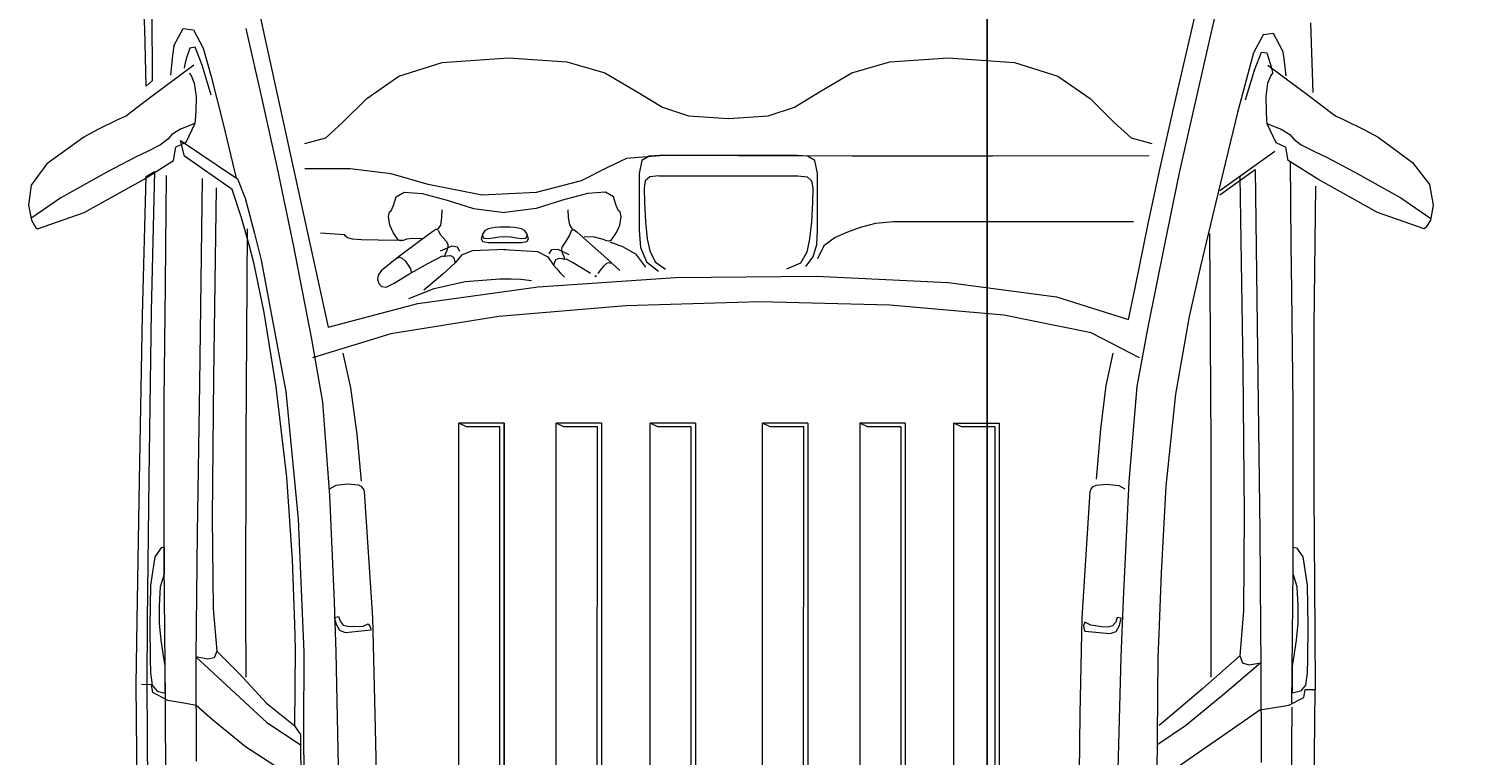
# Model space of a CAD drawing. Units: inches. Extents: x 37 to 706, y -568 to 110.
# Tile 12 of 24: x 449 to 494, y -428 to -405. Entities that reach past the tile are written whole.
import ezdxf

# ---------------------------------------------------------------- set-up
doc = ezdxf.new("R2010")
doc.units = ezdxf.units.IN
doc.header["$MEASUREMENT"] = 0
doc.layers.add('A-ANNO-DIMS', color=2, linetype='Continuous', lineweight=18)
doc.layers.add('A-SITE-VEHI', color=8, linetype='Continuous', lineweight=13)
doc.styles.get("Standard").update_dxf_attribs({"font": 'arial.ttf'})
doc.dimstyles.get("Standard").update_dxf_attribs({"dimtxt": 0.18, "dimasz": 0.18, "dimexe": 0.18, "dimexo": 0.0625, "dimgap": 0.09, "dimtad": 0, "dimtih": 1, "dimtoh": 1, "dimdec": 0, "dimzin": 0, "dimdsep": 46, "dimlunit": 3, "dimtxsty": 'Standard', "dimcen": 0.09, "dimadec": 0, "dimazin": 0, "dimtfac": 1, "dimtdec": 0, "dimtofl": 0, "dimtmove": 0, "dimatfit": 3, "dimfxl": 1, "dimtolj": 1, "dimtzin": 0, "dimarcsym": 0})

# ---------------------------------------------------------------- blocks, each defined once
blk = doc.blocks.new('CAR-SEDAN-PLAN')
for p, q in [((3.672, 63.126), (3.614, 64.361)), ((7.243, 63.902), (9.479, 53.69)), ((36.731, 62.877), (36.956, 63.837)), ((37.632, 64.039), (37.389, 62.984)), ((3.894, 63.679), (3.912, 61.483)), ((3.719, 61.318), (3.672, 63.126)), ((4.598, 62.593), (4.885, 63.135)), ((4.885, 63.135), (5.211, 63.093)), ((5.211, 63.093), (5.522, 62.522)), ((6.866, 63.136), (7.386, 60.866)), ((37.389, 62.984), (36.869, 60.714)), ((39.044, 62.941), (38.733, 62.37)), ((39.37, 62.983), (39.044, 62.941)), ((39.657, 62.441), (39.37, 62.983)), ((40.544, 63.318), (40.611, 61.119)), ((4.598, 62.593), (4.555, 62.29)), ((5.096, 62.522), (4.986, 62.183)), ((5.263, 62.546), (5.096, 62.522)), ((5.485, 61.977), (5.263, 62.546)), ((5.522, 62.522), (5.778, 61.618)), ((36.246, 60.784), (36.731, 62.877)), ((4.555, 62.29), (4.518, 61.981)), ((4.986, 62.183), (4.933, 61.962)), ((11.711, 61.631), (13.079, 62.064)), ((13.079, 62.064), (15.179, 62.211)), ((15.179, 62.211), (17.021, 62.087)), ((17.021, 62.087), (18.221, 61.732)), ((26.04, 61.732), (27.24, 62.087)), ((27.24, 62.087), (29.082, 62.211)), ((29.082, 62.211), (31.182, 62.064)), ((31.182, 62.064), (32.55, 61.631)), ((38.733, 62.37), (38.23, 60.486)), ((38.77, 61.826), (38.993, 62.394)), ((38.993, 62.394), (39.16, 62.37)), ((39.16, 62.37), (39.269, 62.031)), ((39.269, 62.031), (39.323, 61.81)), ((39.657, 62.441), (39.694, 62.178)), ((39.694, 62.178), (39.728, 61.911)), ((5.225, 61.98), (3.867, 60.965)), ((4.518, 61.981), (4.486, 61.667)), ((4.933, 61.962), (4.918, 61.883)), ((5.083, 61.731), (5.138, 61.656)), ((5.138, 61.656), (5.241, 61.415)), ((5.77, 61.03), (5.485, 61.977)), ((5.778, 61.618), (6.153, 60.123)), ((10.694, 60.923), (11.711, 61.631)), ((18.221, 61.732), (19.198, 61.17)), ((25.063, 61.17), (26.04, 61.732)), ((32.55, 61.631), (33.567, 60.923)), ((38.485, 60.879), (38.77, 61.826)), ((39.282, 61.656), (39.179, 61.415)), ((39.195, 61.98), (40.553, 60.965)), ((39.337, 61.731), (39.282, 61.656)), ((39.323, 61.81), (39.337, 61.731)), ((39.728, 61.911), (39.758, 61.639)), ((3.912, 61.483), (3.719, 61.318)), ((5.241, 61.415), (5.296, 60.985)), ((19.198, 61.17), (20.044, 60.65)), ((24.217, 60.65), (25.063, 61.17)), ((39.179, 61.415), (39.124, 60.985)), ((3.867, 60.965), (3.244, 60.496)), ((5.296, 60.985), (5.287, 60.527)), ((7.386, 60.866), (7.866, 58.722)), ((9.94, 60.179), (10.694, 60.923)), ((20.044, 60.65), (20.871, 60.374)), ((23.39, 60.374), (24.217, 60.65)), ((33.567, 60.923), (34.321, 60.179)), ((35.784, 58.735), (36.246, 60.784)), ((36.869, 60.714), (36.389, 58.57)), ((39.124, 60.985), (39.133, 60.527)), ((40.553, 60.965), (41.176, 60.496)), ((2.793, 60.236), (2.192, 59.94)), ((3.094, 60.381), (2.793, 60.236)), ((3.244, 60.496), (3.094, 60.381)), ((5.27, 60.235), (5.26, 60.133)), ((5.287, 60.527), (5.27, 60.235)), ((20.871, 60.374), (22.131, 60.293)), ((22.131, 60.293), (23.39, 60.374)), ((38.23, 60.486), (37.544, 57.648)), ((39.133, 60.527), (39.151, 60.235)), ((39.151, 60.235), (39.16, 60.133)), ((41.176, 60.496), (41.326, 60.381)), ((41.326, 60.381), (41.628, 60.236)), ((41.628, 60.236), (42.229, 59.941)), ((2.192, 59.94), (1.744, 59.706)), ((4.534, 59.788), (4.408, 59.635)), ((4.803, 59.956), (4.534, 59.788)), ((5.26, 60.133), (4.803, 59.956)), ((5.26, 60.133), (4.976, 59.529)), ((6.153, 60.123), (6.566, 58.409)), ((9.397, 59.68), (9.94, 60.179)), ((34.321, 60.179), (34.865, 59.68)), ((39.16, 60.133), (39.444, 59.529)), ((39.16, 60.133), (39.617, 59.956)), ((39.617, 59.956), (39.886, 59.788)), ((39.886, 59.788), (40.012, 59.635)), ((42.229, 59.941), (42.676, 59.706)), ((1.744, 59.706), (0.573, 58.863)), ((4.173, 59.456), (3.756, 59.246)), ((4.408, 59.635), (4.173, 59.456)), ((4.586, 58.96), (4.657, 59.387)), ((4.976, 59.529), (4.657, 59.387)), ((4.806, 59.598), (6.608, 58.388)), ((4.93, 59.103), (4.806, 59.598)), ((8.74, 59.507), (9.397, 59.68)), ((34.865, 59.68), (35.522, 59.507)), ((39.444, 59.529), (39.764, 59.387)), ((39.835, 58.96), (39.764, 59.387)), ((40.012, 59.635), (40.248, 59.456)), ((40.248, 59.456), (40.665, 59.246)), ((42.676, 59.706), (43.766, 58.903)), ((0.573, 58.863), (0.081, 58.181)), ((3.378, 59.067), (2.473, 58.595)), ((3.756, 59.246), (3.378, 59.067)), ((3.652, 58.378), (4.586, 58.96)), ((6.443, 58.044), (4.93, 59.103)), ((18.909, 59.028), (18.306, 58.744)), ((20.089, 59.124), (18.909, 59.028)), ((19.397, 58.963), (19.308, 58.556)), ((19.628, 59.105), (19.397, 58.963)), ((19.948, 59.122), (19.628, 59.105)), ((24.314, 59.122), (19.948, 59.122)), ((22.452, 59.111), (20.089, 59.124)), ((26.04, 59.104), (22.452, 59.111)), ((24.634, 59.105), (24.314, 59.122)), ((24.864, 58.963), (24.634, 59.105)), ((24.953, 58.556), (24.864, 58.963)), ((30.49, 59.105), (26.04, 59.104)), ((35.437, 59.117), (30.49, 59.105)), ((39.408, 59.245), (37.668, 58.002)), ((40.768, 58.378), (39.835, 58.96)), ((39.893, 58.942), (39.907, 57.649)), ((40.665, 59.246), (41.042, 59.067)), ((41.042, 59.067), (41.947, 58.595)), ((43.766, 58.903), (44.299, 58.201)), ((2.473, 58.595), (1.023, 57.787)), ((1.762, 57.317), (3.652, 58.378)), ((3.605, 54.068), (3.719, 58.456)), ((3.719, 58.456), (3.98, 58.613)), ((3.98, 58.613), (3.877, 54.201)), ((4.349, 58.487), (4.338, 57.349)), ((5.491, 58.398), (5.4, 51.914)), ((6.608, 58.388), (6.849, 57.774)), ((7.866, 58.722), (8.367, 56.297)), ((10.166, 58.704), (8.741, 58.704)), ((11.465, 58.539), (10.166, 58.704)), ((12.633, 58.209), (11.465, 58.539)), ((18.306, 58.744), (17.476, 58.319)), ((19.308, 58.556), (19.308, 56.766)), ((19.642, 58.446), (19.501, 58.322)), ((19.929, 58.483), (19.642, 58.446)), ((19.929, 58.483), (24.332, 58.483)), ((24.332, 58.483), (24.619, 58.446)), ((24.619, 58.446), (24.76, 58.322)), ((24.953, 56.766), (24.953, 58.556)), ((35.422, 57.018), (35.784, 58.735)), ((36.389, 58.57), (35.918, 56.312)), ((37.675, 57.879), (38.788, 58.684)), ((38.307, 58.463), (38.397, 52.383)), ((38.788, 58.684), (38.877, 52.125)), ((42.658, 57.317), (40.768, 58.378)), ((41.947, 58.595), (43.397, 57.787)), ((0.081, 58.181), (0, 57.551)), ((5.932, 58.096), (5.844, 52.097)), ((6.733, 57.156), (6.443, 58.044)), ((11.627, 57.82), (11.874, 57.964)), ((11.874, 57.964), (12.448, 57.926)), ((12.448, 57.926), (13.235, 57.705)), ((14.34, 57.866), (12.633, 58.209)), ((16.051, 57.949), (14.34, 57.866)), ((17.476, 58.319), (16.051, 57.949)), ((17.673, 57.926), (16.886, 57.705)), ((18.247, 57.964), (17.673, 57.926)), ((18.494, 57.82), (18.247, 57.964)), ((19.501, 58.322), (19.463, 58.09)), ((19.463, 58.09), (19.473, 57.639)), ((24.76, 58.322), (24.798, 58.09)), ((24.798, 58.09), (24.788, 57.639)), ((40.697, 58.154), (40.647, 53.716)), ((44.299, 58.201), (44.42, 57.551)), ((0, 57.551), (0.089, 57.074)), ((1.023, 57.787), (0.071, 57.125)), ((6.849, 57.774), (7.147, 56.658)), ((11.466, 57.369), (11.535, 57.542)), ((11.535, 57.542), (11.627, 57.82)), ((13.235, 57.705), (14.073, 57.447)), ((16.886, 57.705), (16.048, 57.447)), ((18.587, 57.542), (18.494, 57.82)), ((18.655, 57.369), (18.587, 57.542)), ((19.473, 57.639), (19.505, 57.028)), ((24.788, 57.639), (24.756, 57.028)), ((37.544, 57.648), (37.064, 55.622)), ((39.907, 57.649), (39.918, 56.282)), ((43.397, 57.787), (44.349, 57.125)), ((44.42, 57.551), (44.331, 57.074)), ((0.089, 57.074), (0.218, 56.857)), ((0.284, 56.806), (1.762, 57.317)), ((4.338, 57.349), (4.334, 56.285)), ((6.975, 56.299), (6.733, 57.156)), ((11.38, 57.195), (11.412, 57.338)), ((11.422, 56.921), (11.38, 57.195)), ((11.412, 57.338), (11.466, 57.369)), ((13.059, 57.159), (13.022, 56.924)), ((13.069, 57.405), (13.059, 57.159)), ((14.073, 57.447), (15.061, 57.323)), ((16.048, 57.447), (15.061, 57.323)), ((17.052, 57.405), (17.064, 57.16)), ((17.064, 57.16), (17.104, 56.925)), ((18.71, 57.338), (18.655, 57.369)), ((18.7, 56.921), (18.742, 57.195)), ((18.742, 57.195), (18.71, 57.338)), ((19.505, 57.028), (19.564, 56.492)), ((24.756, 57.028), (24.697, 56.492)), ((27.353, 57.026), (26.785, 56.971)), ((34.947, 57.026), (27.353, 57.026)), ((34.991, 54.942), (35.422, 57.018)), ((44.136, 56.806), (42.658, 57.317)), ((44.331, 57.074), (44.202, 56.857)), ((0.218, 56.857), (0.284, 56.806)), ((6.907, 56.804), (6.866, 50.096)), ((7.147, 56.658), (7.352, 55.813)), ((9.992, 56.613), (9.236, 56.668)), ((10.013, 56.583), (9.992, 56.613)), ((10.09, 56.523), (10.013, 56.583)), ((11.533, 56.687), (11.422, 56.921)), ((11.635, 56.528), (11.533, 56.687)), ((12.786, 56.72), (12.355, 56.402)), ((12.875, 56.778), (12.786, 56.72)), ((12.911, 56.779), (12.875, 56.778)), ((12.917, 56.768), (12.911, 56.779)), ((13.022, 56.924), (12.917, 56.768)), ((12.953, 56.766), (13.019, 56.626)), ((13.019, 56.626), (13.109, 56.514)), ((14.318, 56.49), (14.367, 56.638)), ((14.36, 56.563), (14.367, 56.638)), ((14.415, 56.496), (14.36, 56.563)), ((14.367, 56.638), (14.454, 56.763)), ((14.454, 56.763), (14.547, 56.817)), ((14.547, 56.817), (14.641, 56.839)), ((14.641, 56.839), (14.756, 56.854)), ((14.756, 56.854), (14.903, 56.863)), ((14.903, 56.863), (15.061, 56.866)), ((15.061, 56.866), (15.218, 56.863)), ((15.218, 56.863), (15.366, 56.854)), ((15.366, 56.854), (15.481, 56.839)), ((15.481, 56.839), (15.574, 56.817)), ((15.574, 56.817), (15.668, 56.763)), ((15.668, 56.763), (15.755, 56.638)), ((15.761, 56.563), (15.706, 56.496)), ((15.755, 56.638), (15.804, 56.49)), ((15.755, 56.638), (15.761, 56.563)), ((17.103, 56.601), (17.016, 56.44)), ((17.171, 56.766), (17.103, 56.601)), ((17.104, 56.925), (17.207, 56.766)), ((17.207, 56.766), (17.214, 56.776)), ((17.214, 56.776), (17.249, 56.774)), ((17.249, 56.774), (17.335, 56.711)), ((17.335, 56.711), (17.648, 56.433)), ((18.486, 56.528), (18.589, 56.687)), ((18.589, 56.687), (18.7, 56.921)), ((19.308, 56.766), (19.356, 56.213)), ((24.923, 56.308), (24.953, 56.766)), ((25.895, 56.696), (25.508, 56.53)), ((26.297, 56.842), (25.895, 56.696)), ((26.785, 56.971), (26.297, 56.842)), ((37.348, 56.652), (37.389, 49.984)), ((44.202, 56.857), (44.136, 56.806)), ((4.334, 56.285), (4.314, 54.993)), ((7.131, 55.691), (6.975, 56.299)), ((8.367, 56.297), (8.95, 53.318)), ((10.24, 56.475), (10.09, 56.523)), ((10.531, 56.453), (10.24, 56.475)), ((11.052, 56.441), (10.531, 56.453)), ((11.845, 56.437), (11.052, 56.441)), ((11.702, 56.448), (11.635, 56.528)), ((12.355, 56.402), (11.642, 55.878)), ((11.766, 56.42), (11.702, 56.448)), ((11.845, 56.437), (11.766, 56.42)), ((11.958, 56.473), (11.845, 56.437)), ((12.138, 56.495), (11.958, 56.473)), ((12.421, 56.483), (12.138, 56.495)), ((13.382, 56.251), (13.02, 56.096)), ((13.109, 56.514), (13.201, 56.416)), ((13.223, 56.122), (13.181, 56.026)), ((13.201, 56.416), (13.259, 56.323)), ((13.263, 56.228), (13.223, 56.122)), ((13.259, 56.323), (13.263, 56.228)), ((13.569, 56.226), (13.382, 56.251)), ((13.642, 56.091), (13.569, 56.226)), ((15.088, 56.145), (14.025, 56.105)), ((14.36, 56.396), (14.318, 56.49)), ((14.531, 56.364), (14.36, 56.396)), ((14.531, 56.483), (14.415, 56.496)), ((14.697, 56.511), (14.531, 56.483)), ((15.59, 56.364), (14.531, 56.364)), ((14.885, 56.536), (14.697, 56.511)), ((15.07, 56.547), (14.885, 56.536)), ((15.033, 56.145), (16.092, 56.088)), ((15.249, 56.536), (15.07, 56.547)), ((15.429, 56.511), (15.249, 56.536)), ((15.59, 56.483), (15.429, 56.511)), ((15.706, 56.496), (15.59, 56.483)), ((15.761, 56.396), (15.59, 56.364)), ((15.804, 56.49), (15.761, 56.396)), ((16.467, 56.017), (16.547, 56.148)), ((16.547, 56.148), (16.735, 56.163)), ((16.735, 56.163), (17.089, 55.989)), ((16.862, 56.228), (16.852, 56.134)), ((16.852, 56.134), (16.887, 56.026)), ((16.924, 56.318), (16.862, 56.228)), ((17.016, 56.44), (16.924, 56.318)), ((17.573, 56.556), (17.889, 56.549)), ((17.648, 56.433), (18.193, 55.945)), ((17.889, 56.549), (18.13, 56.492)), ((18.13, 56.492), (18.276, 56.437)), ((18.276, 56.437), (18.355, 56.42)), ((18.355, 56.42), (18.419, 56.448)), ((18.383, 56.393), (18.78, 56.247)), ((18.419, 56.448), (18.486, 56.528)), ((18.78, 56.247), (19.189, 56.016)), ((19.356, 56.213), (19.539, 55.764)), ((19.564, 56.492), (19.646, 56.107)), ((24.697, 56.492), (24.611, 56.07)), ((24.809, 55.915), (24.923, 56.308)), ((25.149, 56.27), (24.945, 55.856)), ((25.508, 56.53), (25.149, 56.27)), ((35.918, 56.312), (35.385, 53.644)), ((39.918, 56.282), (39.941, 54.841)), ((7.449, 54.154), (7.131, 55.691)), ((7.352, 55.813), (8.134, 51.663)), ((11.642, 55.878), (11.149, 55.48)), ((11.673, 55.883), (11.744, 55.903)), ((11.744, 55.903), (11.817, 55.879)), ((11.817, 55.879), (11.906, 55.788)), ((11.906, 55.788), (12.007, 55.658)), ((12.007, 55.658), (12.081, 55.535)), ((12.025, 55.371), (12.63, 55.707)), ((12.63, 55.707), (13.094, 55.946)), ((13.094, 55.946), (13.107, 55.941)), ((13.495, 55.733), (13.1, 55.373)), ((13.107, 55.941), (13.151, 55.937)), ((13.151, 55.937), (13.232, 55.948)), ((13.181, 56.026), (13.168, 55.97)), ((13.168, 55.97), (13.168, 55.951)), ((13.232, 55.948), (13.338, 55.959)), ((13.338, 55.959), (13.435, 55.908)), ((13.435, 55.908), (13.495, 55.733)), ((13.686, 55.974), (13.495, 55.733)), ((14.025, 56.105), (13.686, 55.974)), ((16.092, 56.088), (16.42, 55.921)), ((16.42, 55.921), (16.595, 55.651)), ((16.664, 55.823), (16.595, 55.651)), ((16.764, 55.869), (16.664, 55.823)), ((16.869, 55.852), (16.764, 55.869)), ((16.949, 55.838), (16.869, 55.852)), ((16.887, 56.026), (16.924, 55.928)), ((16.924, 55.928), (16.933, 55.871)), ((16.933, 55.871), (16.933, 55.852)), ((16.993, 55.84), (16.949, 55.838)), ((17.006, 55.843), (16.993, 55.84)), ((17.202, 55.734), (17.006, 55.843)), ((17.461, 55.581), (17.202, 55.734)), ((18.279, 55.71), (18.185, 55.624)), ((18.193, 55.945), (18.694, 55.483)), ((18.352, 55.729), (18.279, 55.71)), ((18.422, 55.706), (18.352, 55.729)), ((19.189, 56.016), (19.512, 55.595)), ((19.539, 55.764), (19.916, 55.467)), ((19.646, 56.107), (19.813, 55.756)), ((19.813, 55.756), (20.146, 55.524)), ((24.411, 55.715), (23.966, 55.531)), ((24.611, 56.07), (24.411, 55.715)), ((24.58, 55.614), (24.809, 55.915)), ((11.052, 55.336), (11.032, 55.197)), ((11.149, 55.48), (11.052, 55.336)), ((11.558, 55.084), (12.025, 55.371)), ((12.081, 55.535), (12.097, 55.422)), ((13.1, 55.373), (12.692, 55.023)), ((13.811, 55.137), (14.905, 55.222)), ((14.905, 55.222), (15.259, 55.221)), ((15.259, 55.221), (15.572, 55.208)), ((15.572, 55.208), (15.9, 55.17)), ((16.11, 54.971), (20.454, 55.259)), ((16.595, 55.651), (16.702, 55.534)), ((16.702, 55.534), (16.812, 55.413)), ((16.812, 55.413), (16.943, 55.271)), ((17.765, 55.393), (17.461, 55.581)), ((17.911, 55.307), (17.963, 55.31)), ((17.928, 55.308), (17.911, 55.307)), ((17.945, 55.309), (17.928, 55.308)), ((17.963, 55.31), (17.945, 55.309)), ((18.053, 55.468), (18.004, 55.394)), ((18.116, 55.545), (18.053, 55.468)), ((18.185, 55.624), (18.116, 55.545)), ((20.454, 55.259), (24.918, 55.306)), ((24.918, 55.306), (29.077, 55.104)), ((37.064, 55.622), (36.708, 54.03)), ((4.314, 54.993), (4.274, 51.392)), ((11.032, 55.197), (11.073, 55.073)), ((11.073, 55.073), (11.161, 54.978)), ((11.161, 54.978), (11.312, 54.961)), ((11.312, 54.961), (11.558, 55.084)), ((12.03, 54.597), (12.826, 54.914)), ((12.31, 54.446), (16.11, 54.971)), ((12.692, 55.023), (12.503, 54.866)), ((12.826, 54.914), (13.811, 55.137)), ((29.077, 55.104), (32.507, 54.649)), ((34.783, 53.934), (34.991, 54.942)), ((39.941, 54.841), (39.982, 51.24)), ((9.479, 53.69), (12.31, 54.446)), ((18.887, 54.369), (14.875, 54.03)), ((23.128, 54.492), (18.887, 54.369)), ((27.235, 54.394), (23.128, 54.492)), ((30.846, 54.07), (27.235, 54.394)), ((32.507, 54.649), (34.783, 53.934)), ((3.505, 48.842), (3.605, 54.068)), ((3.877, 54.201), (3.8, 48.921)), ((7.831, 51.803), (7.449, 54.154)), ((14.875, 54.03), (11.451, 53.479)), ((33.599, 53.515), (30.846, 54.07)), ((36.708, 54.03), (36.272, 51.578)), ((11.451, 53.479), (8.979, 52.723)), ((35.133, 52.723), (33.599, 53.515)), ((35.385, 53.644), (35.049, 51.82)), ((40.647, 53.716), (40.649, 48.459)), ((8.95, 53.318), (9.297, 51.325)), ((9.937, 52.871), (10.178, 51.78)), ((34.292, 52.871), (34.07, 51.849)), ((5.844, 52.097), (5.807, 47.67)), ((38.397, 52.383), (38.441, 47.777)), ((38.877, 52.125), (38.933, 47.216)), ((5.4, 51.914), (5.336, 47.171)), ((8.162, 48.95), (7.831, 51.803)), ((8.134, 51.663), (8.527, 47.62)), ((10.178, 51.78), (10.383, 50.312)), ((34.07, 51.849), (33.895, 50.463)), ((35.049, 51.82), (34.796, 48.812)), ((4.274, 51.392), (4.272, 47.831)), ((9.297, 51.325), (9.518, 48.368)), ((36.272, 51.578), (35.963, 48.661)), ((39.982, 51.24), (39.983, 47.679)), ((10.383, 50.312), (10.515, 48.827)), ((13.846, 50.543), (13.603, 50.661)), ((15.035, 50.661), (13.603, 50.661)), ((13.604, 13.133), (13.604, 50.661)), ((14.905, 50.543), (13.846, 50.543)), ((14.891, 13.73), (14.905, 50.543)), ((15.034, 50.661), (15.034, 13.133)), ((15.035, 50.661), (15.035, 13.133)), ((16.928, 50.543), (16.685, 50.661)), ((18.117, 50.661), (16.685, 50.661)), ((16.686, 13.133), (16.686, 50.661)), ((17.987, 50.543), (16.928, 50.543)), ((17.973, 13.73), (17.987, 50.543)), ((18.115, 50.661), (18.115, 13.133)), ((18.117, 50.661), (18.117, 13.133)), ((19.899, 50.543), (19.656, 50.661)), ((21.088, 50.661), (19.656, 50.661)), ((19.657, 13.133), (19.657, 50.661)), ((20.958, 50.543), (19.899, 50.543)), ((20.944, 13.73), (20.958, 50.543)), ((21.087, 50.661), (21.087, 13.133)), ((21.088, 50.661), (21.088, 13.133)), ((23.454, 50.543), (23.211, 50.661)), ((24.643, 50.661), (23.211, 50.661)), ((23.212, 13.133), (23.212, 50.661)), ((24.513, 50.543), (23.454, 50.543)), ((24.499, 13.73), (24.513, 50.543)), ((24.642, 50.661), (24.642, 13.133)), ((24.643, 50.661), (24.643, 13.133)), ((26.535, 50.543), (26.293, 50.661)), ((27.725, 50.661), (26.293, 50.661)), ((26.294, 13.133), (26.294, 50.661)), ((27.595, 50.543), (26.535, 50.543)), ((27.581, 13.73), (27.595, 50.543)), ((27.723, 50.661), (27.723, 13.133)), ((27.725, 50.661), (27.725, 13.133)), ((29.265, 13.133), (29.265, 50.661)), ((29.508, 50.543), (29.265, 50.661)), ((29.265, 50.661), (30.696, 50.661)), ((30.567, 50.543), (29.508, 50.543)), ((30.553, 13.73), (30.567, 50.543)), ((30.696, 50.661), (30.696, 13.133)), ((33.895, 50.463), (33.764, 48.882)), ((6.866, 50.096), (6.863, 44.784)), ((37.389, 49.984), (37.39, 44.744)), ((3.8, 48.921), (3.752, 44.431)), ((8.341, 46.338), (8.162, 48.95)), ((3.432, 44.406), (3.505, 48.842)), ((9.72, 48.689), (9.523, 48.579)), ((10.096, 48.73), (9.72, 48.689)), ((10.436, 48.697), (10.096, 48.73)), ((10.523, 48.654), (10.436, 48.697)), ((10.593, 48.583), (10.523, 48.654)), ((10.625, 48.497), (10.593, 48.583)), ((10.882, 44.496), (10.625, 48.497)), ((33.322, 44.496), (33.571, 48.497)), ((33.571, 48.497), (33.602, 48.583)), ((33.602, 48.583), (33.672, 48.654)), ((33.672, 48.654), (33.759, 48.697)), ((33.759, 48.697), (34.099, 48.73)), ((34.099, 48.73), (34.475, 48.689)), ((34.475, 48.689), (34.672, 48.579)), ((34.796, 48.812), (34.613, 45.086)), ((35.963, 48.661), (35.82, 45.919)), ((40.649, 48.459), (40.673, 44.07)), ((9.518, 48.368), (9.661, 45.012)), ((4.272, 47.831), (4.279, 46.22)), ((5.807, 47.67), (5.836, 44.794)), ((8.527, 47.62), (8.706, 43.417)), ((38.441, 47.777), (38.417, 44.723)), ((39.983, 47.679), (39.977, 46.068)), ((5.336, 47.171), (5.299, 44.26)), ((38.933, 47.216), (38.963, 44.139)), ((4.192, 46.715), (3.994, 46.427)), ((4.293, 46.735), (4.192, 46.715)), ((4.301, 45.897), (4.293, 46.735)), ((39.989, 45.897), (39.997, 46.735)), ((39.997, 46.735), (40.098, 46.715)), ((40.098, 46.715), (40.296, 46.427)), ((3.994, 46.427), (3.854, 45.534)), ((4.279, 46.22), (4.314, 41.922)), ((8.42, 44.315), (8.341, 46.338)), ((40.296, 46.427), (40.436, 45.534)), ((4.174, 45.486), (4.301, 45.897)), ((35.82, 45.919), (35.739, 43.991)), ((39.977, 46.068), (39.941, 41.77)), ((40.115, 45.486), (39.989, 45.897)), ((3.854, 45.534), (3.83, 44.25)), ((4.14, 44.879), (4.174, 45.486)), ((40.15, 44.879), (40.115, 45.486)), ((40.436, 45.534), (40.46, 44.25)), ((4.141, 44.332), (4.14, 44.879)), ((9.661, 45.012), (9.713, 43.414)), ((34.613, 45.086), (34.542, 43.262)), ((40.149, 44.332), (40.15, 44.879)), ((3.403, 42.392), (3.432, 44.406)), ((3.752, 44.431), (3.734, 42.392)), ((5.836, 44.794), (5.948, 43.449)), ((6.863, 44.784), (6.869, 42.622)), ((9.676, 44.516), (9.798, 44.542)), ((9.733, 44.29), (9.676, 44.516)), ((9.798, 44.542), (9.85, 44.396)), ((9.85, 44.396), (9.949, 44.274)), ((10.962, 41.449), (10.882, 44.496)), ((33.258, 41.449), (33.322, 44.496)), ((33.404, 44.362), (33.363, 44.248)), ((33.591, 44.267), (33.404, 44.362)), ((34.379, 44.368), (34.28, 44.247)), ((34.431, 44.514), (34.379, 44.368)), ((34.554, 44.489), (34.431, 44.514)), ((34.496, 44.262), (34.554, 44.489)), ((37.39, 44.744), (37.384, 42.623)), ((38.417, 44.723), (38.307, 43.297)), ((3.83, 44.25), (3.844, 43.196)), ((4.188, 43.792), (4.141, 44.332)), ((5.299, 44.26), (5.287, 43.269)), ((8.437, 43.503), (8.42, 44.315)), ((9.838, 44.098), (9.733, 44.29)), ((10.025, 44.031), (9.838, 44.098)), ((9.949, 44.274), (10.095, 44.234)), ((10.824, 44.11), (10.025, 44.031)), ((10.095, 44.234), (10.264, 44.226)), ((10.264, 44.226), (10.577, 44.234)), ((10.577, 44.234), (10.743, 44.307)), ((10.743, 44.307), (10.805, 44.214)), ((10.805, 44.214), (10.824, 44.14)), ((10.824, 44.14), (10.824, 44.11)), ((33.363, 44.248), (33.384, 44.134)), ((33.384, 44.134), (33.405, 44.082)), ((33.405, 44.082), (34.204, 44.004)), ((33.943, 44.22), (33.591, 44.267)), ((34.134, 44.207), (33.943, 44.22)), ((34.28, 44.247), (34.134, 44.207)), ((34.204, 44.004), (34.391, 44.071)), ((34.391, 44.071), (34.496, 44.262)), ((35.739, 43.991), (35.714, 43.262)), ((38.963, 44.139), (38.971, 43.074)), ((40.102, 43.792), (40.149, 44.332)), ((40.46, 44.25), (40.446, 43.196)), ((40.673, 44.07), (40.687, 42.232)), ((4.273, 43.24), (4.188, 43.792)), ((5.948, 43.449), (5.871, 43.237)), ((5.948, 43.449), (6.66, 42.737)), ((8.416, 41.085), (8.437, 43.503)), ((40.017, 43.24), (40.102, 43.792)), ((3.844, 43.196), (3.857, 42.759)), ((4.32, 42.987), (4.273, 43.24)), ((4.32, 42.116), (4.32, 42.987)), ((5.287, 43.269), (6.407, 42.232)), ((5.672, 43.197), (5.287, 43.269)), ((5.287, 43.269), (5.301, 39.967)), ((5.871, 43.237), (5.672, 43.197)), ((8.706, 43.417), (8.689, 40.947)), ((9.713, 43.414), (9.796, 39.289)), ((34.542, 43.262), (34.438, 39.318)), ((35.714, 43.262), (35.681, 39.496)), ((38.307, 43.297), (37.13, 42.261)), ((38.971, 43.074), (37.772, 42.057)), ((38.307, 43.297), (38.385, 43.074)), ((38.385, 43.074), (38.586, 43.013)), ((38.586, 43.013), (38.971, 43.074)), ((38.971, 43.074), (38.982, 39.925)), ((39.97, 42.987), (40.017, 43.24)), ((39.97, 42.116), (39.97, 42.987)), ((40.446, 43.196), (40.433, 42.759)), ((3.857, 42.759), (3.913, 42.374)), ((6.66, 42.737), (7.526, 41.803)), ((40.433, 42.759), (40.377, 42.374)), ((3.432, 39.004), (3.403, 42.392)), ((3.888, 42.384), (3.568, 42.392)), ((3.734, 42.392), (3.762, 39.007)), ((3.924, 42.135), (3.888, 42.384)), ((3.913, 42.374), (4.061, 42.185)), ((4.399, 41.888), (3.924, 42.135)), ((4.061, 42.185), (4.32, 42.116)), ((6.407, 42.232), (7.533, 41.191)), ((37.13, 42.261), (36.157, 41.433)), ((40.229, 42.185), (39.97, 42.116)), ((40.377, 42.374), (40.229, 42.185)), ((40.332, 41.983), (40.367, 42.232)), ((40.367, 42.232), (40.674, 42.232)), ((40.658, 38.847), (40.687, 42.232)), ((4.314, 41.922), (4.342, 36.731)), ((4.968, 41.787), (4.399, 41.888)), ((5.301, 41.728), (4.968, 41.787)), ((5.819, 41.275), (5.301, 41.728)), ((7.526, 41.803), (8.416, 41.085)), ((37.772, 42.057), (36.584, 41.081)), ((38.936, 41.591), (39.274, 41.645)), ((39.274, 41.645), (39.851, 41.74)), ((39.851, 41.74), (40.332, 41.983)), ((39.946, 41.674), (39.918, 36.482)), ((6.86, 40.42), (5.819, 41.275)), ((7.533, 41.191), (8.616, 40.477)), ((10.998, 39.61), (10.962, 41.449)), ((33.232, 39.61), (33.258, 41.449)), ((36.157, 41.433), (35.752, 41.094)), ((38.211, 41.09), (38.936, 41.591)), ((8.61, 40.812), (8.416, 41.085)), ((8.623, 38.413), (8.61, 40.812)), ((8.689, 40.947), (8.707, 39.376)), ((36.584, 41.081), (35.717, 40.49)), ((36.975, 40.234), (38.211, 41.09)), ((7.97, 39.706), (6.86, 40.42)), ((36.321, 39.78), (36.975, 40.234))]:
    blk.add_line(p, q)
blk = doc.blocks.new('*D63')
at = {"layer": 'A-ANNO-DIMS', "color": 0, "lineweight": -2, "transparency": 16777216}
for p, q in [((478.958, -142.771), (478.958, -567.638)), ((502.958, -151.771), (502.958, -567.638)), ((479.138, -567.458), (490.628, -567.458)), ((502.778, -567.458), (491.289, -567.458))]:
    blk.add_line(p, q, dxfattribs=at)
at = {"layer": 'A-ANNO-DIMS', "color": 0, "transparency": 16777216}
for points in [[(479.138, -567.428), (479.138, -567.488), (478.958, -567.458)], [(502.778, -567.428), (502.778, -567.488), (502.958, -567.458)]]:
    blk.add_solid(points, dxfattribs=at)
at = {"layer": 'Defpoints', "color": 0, "transparency": 16777216}
for p in [(478.958, -142.708), (502.958, -151.708), (502.958, -567.458)]:
    blk.add_point(p, dxfattribs=at)
at = {"layer": 'A-ANNO-DIMS', "color": 0, "transparency": 16777216, "insert": (490.958, -567.458), "char_height": 0.18, "attachment_point": 5}
blk.add_mtext('\\A1;2\'-0"', dxfattribs=at)

msp = doc.modelspace()

# ---------------------------------------------------------------- block references
at = {"layer": 'A-SITE-VEHI'}
msp.add_blockref('CAR-SEDAN-PLAN', (448.648, -467.674), dxfattribs=at)

# ---------------------------------------------------------------- dimensions: what is measured, and where the dimension line sits
at = {"layer": 'A-ANNO-DIMS'}
dim = msp.add_linear_dim(base=(502.958, -567.458), p1=(478.958, -142.708), p2=(502.958, -151.708), dimstyle='Standard', override={"dimdec": 1, "dimlfac": 1, "dimrnd": 0, "dimzin": 1, "dimdsep": 46, "dimlunit": 4, "dimfrac": 2}, dxfattribs=at)
dim.commit()
dim.dimension.update_dxf_attribs({"geometry": '*D63', "text_midpoint": (490.958, -567.458)})

doc.saveas('drawing.dxf')
